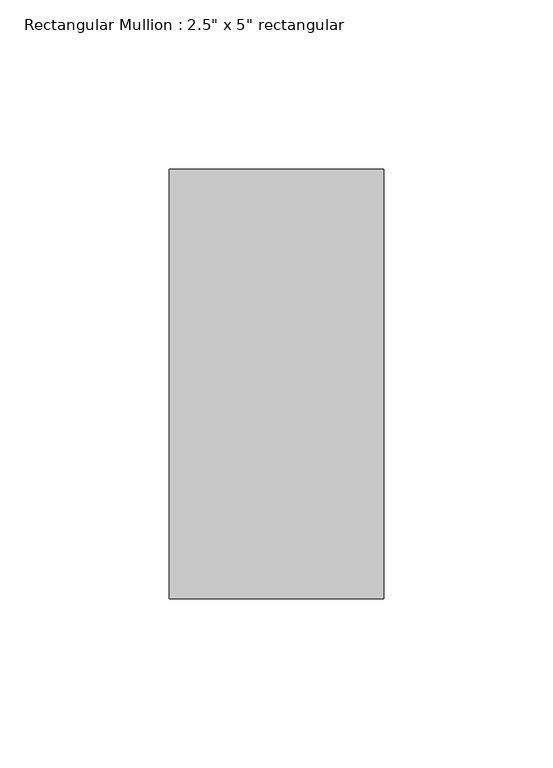
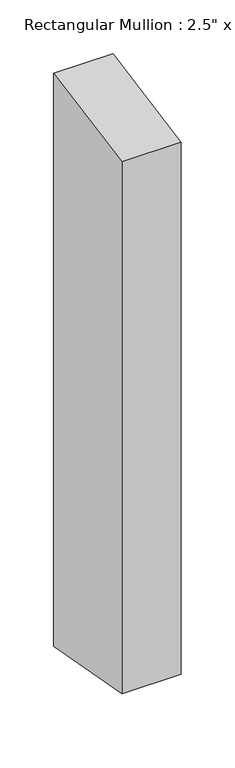
"""IFC4 building model written with IfcOpenShell, lengths in millimetres: member geometry."""

from ifc_helpers import new_model, si_unit, frame, origin, place, context, project, spatial, polyline, outline, extrude, source, transform, mapped, element, save


def member_fe018dc2(model_context):
    return source(origin(), model_context, "Body", "SweptSolid", [
        extrude(outline(polyline([(-63.5, -11.6039351), (63.5, 11.6039351), (63.5, -637.4452824), (-63.5, -614.2374121), (-63.5, -11.6039351)])), frame((-63.5, 0.0, 0.0), z_axis=(1.0, 0.0, 0.0), x_axis=(0.0, 1.0, 0.0)), (0.0, 0.0, 1.0), 63.5),
    ])


if __name__ == "__main__":
    model = new_model("IFC4")
    model_context = context("Model", 3, world=origin())
    ifc_project = project(units=[si_unit("LENGTHUNIT", "METRE", prefix="MILLI")], contexts=[model_context])
    site = spatial("IfcSite", under=ifc_project)
    building = spatial("IfcBuilding", under=site)
    placement = place(None, origin())
    member_shape = member_fe018dc2(model_context)
    element("IfcMember", 1, ObjectType="Rectangular Mullion : 2.5\" x 5\" rectangular", at=placement, inside=building, context=model_context, shape_type="MappedRepresentation", body=[
        mapped(member_shape, transform((0.0, 0.0, 0.0), x_axis=(1.0, 0.0, 0.0), y_axis=(0.0, 1.0, 0.0), z_axis=(0.0, 0.0, 1.0))),
    ])
    save(model, "model.ifc")

# Revit data of these elements
# Type "Rectangular Mullion : 2.5\" x 5\" rectangular"
#   built-in parameter 1007304 = 0.416667 (stored number, unit not read)
#   built-in parameter 1007301 = 0.104167 (stored number, unit not read)
#   built-in parameter 1007300 = 0.104167 (stored number, unit not read)
# Element 1 (IfcMember, "Rectangular Mullion : 2.5\" x 5\" rectangular")
#   Materials on its faces: "Iron, Ductile"
# Materials
#   "Iron, Ductile": class "Metal", colour RGB 0 0 0, transparency 0, Description = "Ductile cast iron", Cost = 0
